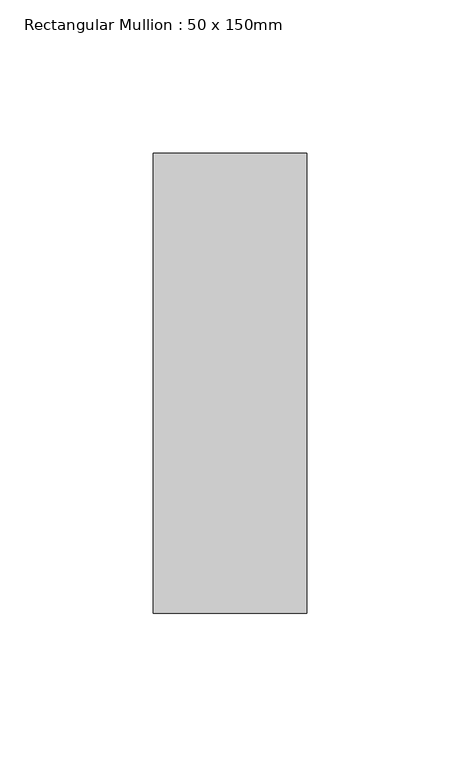
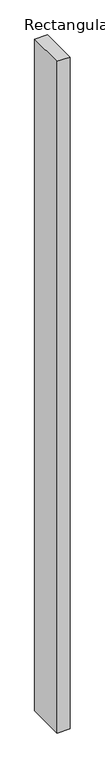
"""IFC4 building model written with IfcOpenShell, lengths in millimetres: member geometry, Rectangular Mullion : 50 x 150mm."""

from ifc_helpers import new_model, si_unit, frame, origin, place, context, project, spatial, polyline, outline, extrude, source, transform, mapped, element, save


def rectangular_mullion_50_x_150mm_bcca0aad(model_context):
    return source(origin(), model_context, "Body", "SweptSolid", [
        extrude(outline(polyline([(25.0, 75.0), (25.0, -75.0), (-25.0, -75.0), (-25.0, 75.0), (25.0, 75.0)])), frame((0.0, 0.0, -2743.2), z_axis=(0.0, 0.0, 1.0), x_axis=(1.0, 0.0, 0.0)), (0.0, 0.0, 1.0), 2743.2),
    ])


if __name__ == "__main__":
    model = new_model("IFC4")
    model_context = context("Model", 3, world=origin())
    ifc_project = project(units=[si_unit("LENGTHUNIT", "METRE", prefix="MILLI")], contexts=[model_context])
    site = spatial("IfcSite", under=ifc_project)
    building = spatial("IfcBuilding", under=site)
    placement = place(None, origin())
    rectangular_mullion_50_x_150mm_shape = rectangular_mullion_50_x_150mm_bcca0aad(model_context)
    element("IfcMember", 1, ObjectType="Rectangular Mullion : 50 x 150mm", at=placement, inside=building, context=model_context, shape_type="MappedRepresentation", body=[
        mapped(rectangular_mullion_50_x_150mm_shape, transform((0.0, 0.0, 0.0), x_axis=(1.0, 0.0, 0.0), y_axis=(0.0, 1.0, 0.0), z_axis=(0.0, 0.0, 1.0))),
    ])
    save(model, "model.ifc")

# Revit data of these elements
# Type "Rectangular Mullion : 50 x 150mm"
#   built-in parameter 1007304 = 0.492126 (stored number, unit not read)
#   built-in parameter 1007301 = 0.082021 (stored number, unit not read)
#   built-in parameter 1007300 = 0.082021 (stored number, unit not read)
# Element 1 (IfcMember, "Rectangular Mullion : 50 x 150mm")
#   Materials on its faces: "Aluminium"
# Materials
#   "Aluminium": class "Metal", colour RGB 247 247 247, transparency 0, Description = "Aluminium 6061", Cost = 0
